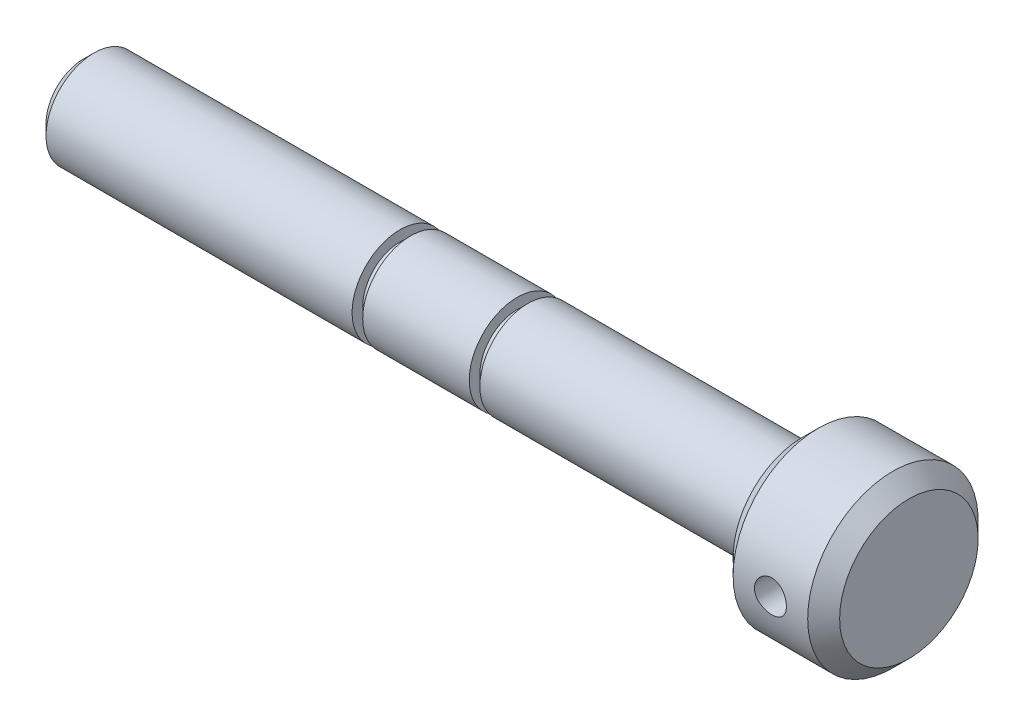
SolidWorks part; units mm, degrees
material "Plain Carbon Steel"
ref_plane "Front Plane" through (0, 0, 0) normal (0, 0, 1) x (1, 0, 0)
ref_plane "Top Plane" through (0, 0, 0) normal (0, 1, 0) x (1, 0, 0)
ref_plane "Right Plane" through (0, 0, 0) normal (1, 0, 0) x (0, 0, -1)
sketch "Bolt Profile Sketch" plane through (0, 0, 0) normal (0, 0, 1) x (1, 0, 0)
  line L0 (0, 0) -> (155, 0) construction
  line L1 (155, 0) -> (155, 16)
  line L2 (155, 16) -> (135, 16)
  line L3 (135, 16) -> (135, 9)
  line L4 (135, 9) -> (83.46, 9)
  line L5 (83.46, 9) -> (83.46, 7)
  line L6 (83.46, 7) -> (81.46, 7)
  line L7 (81.46, 7) -> (81.46, 9)
  line L8 (81.46, 9) -> (61.46, 9)
  line L9 (61.46, 9) -> (61.46, 7)
  line L10 (61.46, 7) -> (59.46, 7)
  line L11 (59.46, 7) -> (59.46, 9)
  line L12 (59.46, 9) -> (0, 9)
  line L13 (0, 9) -> (0, 0)
  line L14 (0, 0) -> (155, 0)
  dimension "D1" = 16
  dimension "D2" = 20
  dimension "D3" = 51.54
  dimension "D4" = 155
  dimension "D5" = 7
  dimension "D6" = 2
  dimension "D7" = 20
  dimension "D8" = 9
  dimension "D9" = 2
revolve "Bolt Body Revolve" add sketch "Bolt Profile Sketch" angle 360 about L0
cosmetic thread "Cosmetic Thread2" parameters "D2"=15.252
chamfer "Head Chamfer 3mm" distance 3 angle 45 2 edges at (155, 0, 16) (135, 0, 16)
chamfer "Edge Chamfer 2mm" distance 2 angle 45 1 edges at (0, 0, 9)
cosmetic thread "Cosmetic Thread1" parameters "D2"=15.252
sketch "Cross Hole Sketch" plane through (0, 0, 0) normal (0, 0, 1) x (1, 0, 0)
  line L0 (155, -13) -> (155, 13) construction
  circle A0 centre (145, 0) radius 3
  dimension "D1" = 6
  dimension "D2" = 10
extrude "Head Cross Hole" cut sketch "Cross Hole Sketch" against normal through all both and the other way through all
